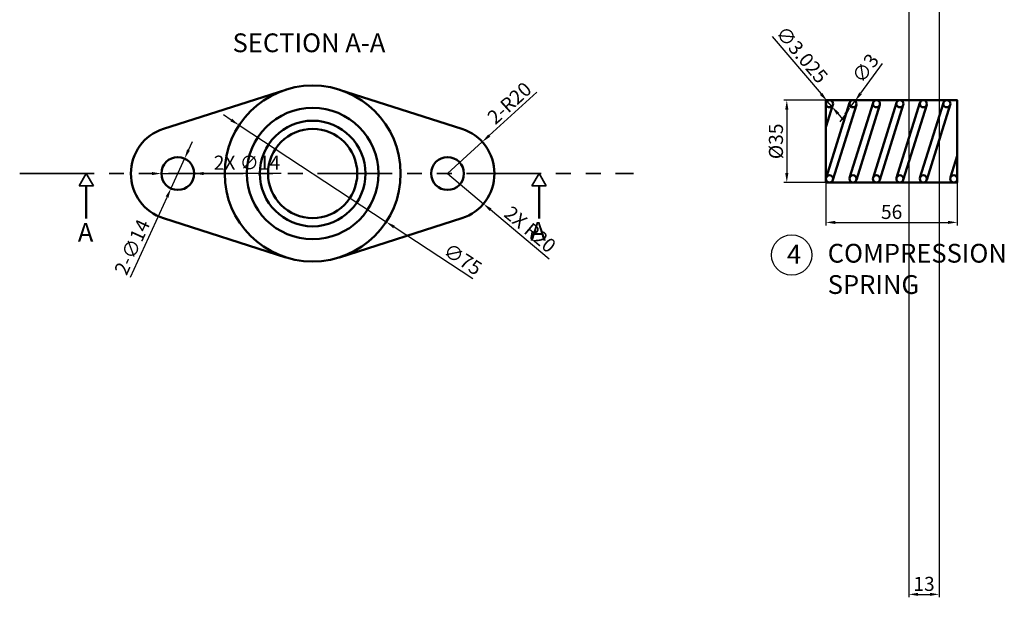
# Model space of a CAD drawing. Units: millimetres. Extents: x 4194 to 4882, y 3816 to 4286.
# Tile 1 of 3: x 4194 to 4614, y 3816 to 4062. Entities that reach past the tile are written whole.
import ezdxf

# ---------------------------------------------------------------- set-up
doc = ezdxf.new("R2010")
doc.units = ezdxf.units.MM
doc.linetypes.add('PHANTOM', pattern=[63.5, 31.75, -6.35, 6.35, -6.35, 6.35, -6.35])
for name, color, linetype, lineweight in [('M-DIMS', 2, 'Continuous', 25), ('M-OUTL', 7, 'Continuous', 50), ('M-SECT', 6, 'PHANTOM', 35), ('M-TEXT', 3, 'Continuous', 25)]:
    doc.layers.add(name, color=color, linetype=linetype, lineweight=lineweight)
doc.styles.get("Standard").update_dxf_attribs({"font": 'arial.ttf'})
doc.dimstyles.new('ISO-25', dxfattribs={"dimtxt": 6, "dimasz": 4, "dimexe": 1.25, "dimexo": 0.625, "dimtad": 1, "dimdec": 0, "dimtxsty": 'Standard', "dimcen": 2.5, "dimadec": 0, "dimazin": 0, "dimtfac": 1, "dimtdec": 0, "dimtmove": 0, "dimatfit": 3, "dimfxl": 1, "dimarcsym": 0})

# ---------------------------------------------------------------- blocks, each defined once
blk = doc.blocks.new('*D5')
at = {"layer": 'Defpoints', "color": 0, "transparency": 16777216}
for p in [(4264.77, 4003.28), (4258.94, 3990.55)]:
    blk.add_point(p, dxfattribs=at)
at = {"layer": 'M-DIMS', "color": 0, "lineweight": -2, "transparency": 16777216}
for p, q in [((4266.44, 4006.92), (4268.1, 4010.55)), ((4264.77, 4003.28), (4258.94, 3990.55)), ((4241.67, 3952.8), (4257.28, 3986.91))]:
    blk.add_line(p, q, dxfattribs=at)
at = {"layer": 'M-DIMS', "color": 0, "transparency": 16777216}
for points in [[(4265.83, 4007.19), (4267.04, 4006.64), (4264.77, 4003.28)], [(4256.67, 3987.19), (4257.89, 3986.63), (4258.94, 3990.55)]]:
    blk.add_solid(points, dxfattribs=at)
at = {"layer": 'M-DIMS', "color": 0, "transparency": 16777216, "insert": (4243.13, 3965.27), "char_height": 6, "attachment_point": 5, "rotation": 65.4036}
blk.add_mtext('2-∅14', dxfattribs=at)
blk = doc.blocks.new('*D6')
at = {"layer": 'Defpoints', "color": 0, "transparency": 16777216}
for p in [(4391.65, 4010.38), (4376.86, 3996.91)]:
    blk.add_point(p, dxfattribs=at)
at = {"layer": 'M-DIMS', "color": 0, "lineweight": -2, "transparency": 16777216}
for p, q in [((4414.9, 4031.53), (4394.61, 4013.07)), ((4376.86, 3996.91), (4391.65, 4010.38))]:
    blk.add_line(p, q, dxfattribs=at)
at = {"layer": 'M-DIMS', "color": 0, "transparency": 16777216}
blk.add_solid([(4394.16, 4013.56), (4395.06, 4012.57), (4391.65, 4010.38)], dxfattribs=at)
at = {"layer": 'M-DIMS', "color": 0, "transparency": 16777216, "insert": (4403.75, 4026.37), "char_height": 6, "attachment_point": 5, "rotation": 42.3036}
blk.add_mtext('2-R20', dxfattribs=at)
blk = doc.blocks.new('*D7')
at = {"layer": 'Defpoints', "color": 0, "transparency": 16777216}
for p in [(4288.01, 4017.5), (4350.7, 3976.33)]:
    blk.add_point(p, dxfattribs=at)
at = {"layer": 'M-DIMS', "color": 0, "lineweight": -2, "transparency": 16777216}
for p, q in [((4284.67, 4019.69), (4281.33, 4021.89)), ((4288.01, 4017.5), (4350.7, 3976.33)), ((4387.68, 3952.05), (4354.05, 3974.13))]:
    blk.add_line(p, q, dxfattribs=at)
at = {"layer": 'M-DIMS', "color": 0, "transparency": 16777216}
for points in [[(4285.04, 4020.25), (4284.3, 4019.14), (4288.01, 4017.5)], [(4354.41, 3974.69), (4353.68, 3973.58), (4350.7, 3976.33)]]:
    blk.add_solid(points, dxfattribs=at)
at = {"layer": 'M-DIMS', "color": 0, "transparency": 16777216, "insert": (4382.93, 3959.78), "char_height": 6, "attachment_point": 5, "rotation": 326.7072}
blk.add_mtext('∅75', dxfattribs=at)
blk = doc.blocks.new('*D30')
at = {"layer": 'Defpoints', "color": 0, "transparency": 16777216}
for p in [(4546.41, 4028.13), (4521.47, 3993.13), (4544.98, 3993.13)]:
    blk.add_point(p, dxfattribs=at)
at = {"layer": 'M-DIMS', "color": 0, "lineweight": -2, "transparency": 16777216}
for p, q in [((4545.79, 4028.13), (4520.22, 4028.13)), ((4521.47, 4024.13), (4521.47, 3997.13)), ((4544.35, 3993.13), (4520.22, 3993.13))]:
    blk.add_line(p, q, dxfattribs=at)
at = {"layer": 'M-DIMS', "color": 0, "transparency": 16777216}
for points in [[(4520.8, 4024.13), (4522.14, 4024.13), (4521.47, 4028.13)], [(4520.8, 3997.13), (4522.14, 3997.13), (4521.47, 3993.13)]]:
    blk.add_solid(points, dxfattribs=at)
at = {"layer": 'M-DIMS', "color": 0, "transparency": 16777216, "insert": (4517.62, 4010.63), "char_height": 6, "attachment_point": 5, "rotation": 90}
blk.add_mtext('%%C35', dxfattribs=at)
blk = doc.blocks.new('*D31')
at = {"layer": 'Defpoints', "color": 0, "transparency": 16777216}
for p in [(4594.15, 4010.63), (4538.15, 4007.59), (4594.15, 3976.09)]:
    blk.add_point(p, dxfattribs=at)
at = {"layer": 'M-DIMS', "color": 0, "lineweight": -2, "transparency": 16777216}
for p, q in [((4594.15, 4010.01), (4594.15, 3974.84)), ((4538.15, 4006.97), (4538.15, 3974.84)), ((4542.15, 3976.09), (4590.15, 3976.09))]:
    blk.add_line(p, q, dxfattribs=at)
at = {"layer": 'M-DIMS', "color": 0, "transparency": 16777216}
for points in [[(4542.15, 3976.76), (4542.15, 3975.42), (4538.15, 3976.09)], [(4590.15, 3976.76), (4590.15, 3975.42), (4594.15, 3976.09)]]:
    blk.add_solid(points, dxfattribs=at)
at = {"layer": 'M-DIMS', "color": 0, "transparency": 16777216, "insert": (4566.15, 3979.78), "char_height": 6, "attachment_point": 5}
blk.add_mtext('56', dxfattribs=at)
blk = doc.blocks.new('*D32')
at = {"layer": 'Defpoints', "color": 0, "transparency": 16777216}
for p in [(4548.78, 4025.41), (4550.56, 4027.85)]:
    blk.add_point(p, dxfattribs=at)
at = {"layer": 'M-DIMS', "color": 0, "lineweight": -2, "transparency": 16777216}
for p, q in [((4562.16, 4043.79), (4552.91, 4031.09)), ((4548.78, 4025.41), (4550.56, 4027.85)), ((4546.42, 4022.18), (4544.07, 4018.94))]:
    blk.add_line(p, q, dxfattribs=at)
at = {"layer": 'M-DIMS', "color": 0, "transparency": 16777216}
for points in [[(4552.37, 4031.48), (4553.45, 4030.69), (4550.56, 4027.85)], [(4545.88, 4022.57), (4546.96, 4021.78), (4548.78, 4025.41)]]:
    blk.add_solid(points, dxfattribs=at)
at = {"layer": 'M-DIMS', "color": 0, "transparency": 16777216, "insert": (4555.6, 4041.32), "char_height": 6, "attachment_point": 5, "rotation": 53.9324}
blk.add_mtext('∅3', dxfattribs=at)
blk = doc.blocks.new('SECTION-ARROW')
for p, q in [((3.04, 5.26), (0, 0)), ((3.04, 5.26), (6.07, 0)), ((6.07, 0), (0, 0))]:
    blk.add_line(p, q)
blk = doc.blocks.new('*D52')
at = {"layer": 'Defpoints', "color": 0, "transparency": 16777216}
for p in [(4586.46, 4107.44), (4573.46, 4094.44), (4586.46, 3817.63)]:
    blk.add_point(p, dxfattribs=at)
at = {"layer": 'M-DIMS', "color": 0, "lineweight": -2, "transparency": 16777216}
for p, q in [((4586.46, 4106.81), (4586.46, 3816.38)), ((4573.46, 4093.81), (4573.46, 3816.38)), ((4577.46, 3817.63), (4582.46, 3817.63))]:
    blk.add_line(p, q, dxfattribs=at)
at = {"layer": 'M-DIMS', "color": 0, "transparency": 16777216}
for points in [[(4577.46, 3818.3), (4577.46, 3816.97), (4573.46, 3817.63)], [(4582.46, 3818.3), (4582.46, 3816.97), (4586.46, 3817.63)]]:
    blk.add_solid(points, dxfattribs=at)
at = {"layer": 'M-DIMS', "color": 0, "transparency": 16777216, "insert": (4579.96, 3821.32), "char_height": 6, "attachment_point": 5}
blk.add_mtext('13', dxfattribs=at)
blk = doc.blocks.new('*D53')
at = {"layer": 'Defpoints', "color": 0, "transparency": 16777216}
for p in [(4376.86, 3996.91), (4392.16, 3984.03)]:
    blk.add_point(p, dxfattribs=at)
at = {"layer": 'M-DIMS', "color": 0, "lineweight": -2, "transparency": 16777216}
for p, q in [((4376.86, 3996.91), (4392.16, 3984.03)), ((4420.13, 3960.49), (4395.22, 3981.46))]:
    blk.add_line(p, q, dxfattribs=at)
at = {"layer": 'M-DIMS', "color": 0, "transparency": 16777216}
blk.add_solid([(4395.65, 3981.97), (4394.79, 3980.95), (4392.16, 3984.03)], dxfattribs=at)
at = {"layer": 'M-DIMS', "color": 0, "transparency": 16777216, "insert": (4411.58, 3972.51), "char_height": 6, "attachment_point": 5, "rotation": 319.9113}
blk.add_mtext('2X R20', dxfattribs=at)
blk = doc.blocks.new('*D54')
at = {"layer": 'Defpoints', "color": 0, "transparency": 16777216}
for p in [(4254.86, 3996.91), (4268.86, 3996.91)]:
    blk.add_point(p, dxfattribs=at)
at = {"layer": 'M-DIMS', "color": 0, "lineweight": -2, "transparency": 16777216}
for p, q in [((4250.86, 3996.91), (4246.86, 3996.91)), ((4254.86, 3996.91), (4268.86, 3996.91)), ((4305.88, 3996.91), (4272.86, 3996.91))]:
    blk.add_line(p, q, dxfattribs=at)
at = {"layer": 'M-DIMS', "color": 0, "transparency": 16777216}
for points in [[(4250.86, 3997.58), (4250.86, 3996.25), (4254.86, 3996.91)], [(4272.86, 3997.58), (4272.86, 3996.25), (4268.86, 3996.91)]]:
    blk.add_solid(points, dxfattribs=at)
at = {"layer": 'M-DIMS', "color": 0, "transparency": 16777216, "insert": (4291.37, 4000.77), "char_height": 6, "attachment_point": 5, "rotation": 359.9997}
blk.add_mtext('2X ∅14', dxfattribs=at)
blk = doc.blocks.new('*D57')
at = {"layer": 'Defpoints', "color": 0, "transparency": 16777216}
for p in [(4538.69, 4027.78), (4540.65, 4025.48)]:
    blk.add_point(p, dxfattribs=at)
at = {"layer": 'M-DIMS', "color": 0, "lineweight": -2, "transparency": 16777216}
for p, q in [((4515.29, 4055.23), (4536.09, 4030.83)), ((4540.65, 4025.48), (4538.69, 4027.78)), ((4543.24, 4022.44), (4545.84, 4019.39))]:
    blk.add_line(p, q, dxfattribs=at)
at = {"layer": 'M-DIMS', "color": 0, "transparency": 16777216}
for points in [[(4536.6, 4031.26), (4535.58, 4030.39), (4538.69, 4027.78)], [(4543.75, 4022.87), (4542.74, 4022), (4540.65, 4025.48)]]:
    blk.add_solid(points, dxfattribs=at)
at = {"layer": 'M-DIMS', "color": 0, "transparency": 16777216, "insert": (4527.33, 4047.05), "char_height": 6, "attachment_point": 5, "rotation": 310.4453}
blk.add_mtext('∅3.025', dxfattribs=at)

msp = doc.modelspace()

# ---------------------------------------------------------------- linework, layer by layer
at = {"layer": 'M-OUTL'}
for p, q in [((4307.9449, 4032.6351), (4255.771, 4015.9653)), ((4330.771, 4032.6351), (4382.9449, 4015.9653)), ((4538.2229, 4027.0821), (4538.1542, 4026.862)), ((4541.1104, 4026.1807), (4538.1542, 4016.711)), ((4548.2229, 4027.0821), (4538.2375, 3995.0945)), ((4551.1104, 4026.1807), (4541.1249, 3994.1931)), ((4558.2229, 4027.0821), (4548.2375, 3995.0945)), ((4561.1104, 4026.1807), (4551.1249, 3994.1931)), ((4568.2229, 4027.0821), (4558.2375, 3995.0945)), ((4571.1104, 4026.1807), (4561.1249, 3994.1931)), ((4578.2229, 4027.0821), (4568.2375, 3995.0945)), ((4581.1104, 4026.1807), (4571.1249, 3994.1931)), ((4588.2229, 4027.0821), (4578.2375, 3995.0945)), ((4591.1104, 4026.1807), (4581.1249, 3994.1931)), ((4591.287, 3995.3159), (4594.1542, 4004.501)), ((4222.8708, 3991.6564), (4222.8708, 3977.7143)), ((4415.8451, 3991.6564), (4415.8451, 3977.7143)), ((4307.9449, 3961.193), (4255.771, 3977.8628)), ((4330.771, 3961.193), (4382.9449, 3977.8628))]:
    msp.add_line(p, q, dxfattribs=at)
msp.add_lwpolyline([(4538.1542, 4028.1314), (4594.1542, 4028.1314), (4594.1542, 3993.1314), (4538.1542, 3993.1314)], close=True, dxfattribs=at)
for centre, radius in [((4319.358, 3996.914), 37.5), ((4539.6667, 4026.6314), 1.5124), ((4549.6667, 4026.6314), 1.5124), ((4559.6667, 4026.6314), 1.5124), ((4569.6667, 4026.6314), 1.5124), ((4579.6667, 4026.6314), 1.5124), ((4589.6667, 4026.6314), 1.5124), ((4319.358, 3996.914), 28), ((4319.358, 3996.914), 22.5), ((4319.358, 3996.914), 19), ((4261.858, 3996.914), 7), ((4376.858, 3996.914), 7), ((4539.6812, 3994.6438), 1.5124), ((4549.6812, 3994.6438), 1.5124), ((4559.6812, 3994.6438), 1.5124), ((4569.6812, 3994.6438), 1.5124), ((4579.6812, 3994.6438), 1.5124), ((4592.6418, 3994.6438), 1.5124)]:
    msp.add_circle(centre, radius, dxfattribs=at)
for centre, radius, start, end in [((4539.6667, 4026.6314), 1.5124, 342.663423, 180), ((4261.858, 3996.914), 20, 107.718932, 252.281068), ((4376.858, 3996.914), 20, 287.718932, 72.281068)]:
    msp.add_arc(centre, radius, start, end, dxfattribs=at)
at = {"layer": 'M-SECT'}
msp.add_line((4194.4762, 3996.914), (4456.1273, 3996.914), dxfattribs=at)
at = {"layer": 'M-TEXT'}
msp.add_circle((4523.548, 3962.2066), 8.6164, dxfattribs=at)

# ---------------------------------------------------------------- block references
at = {"layer": 'M-SECT', "rotation": 119.9999999999872}
msp.add_blockref('SECTION-ARROW', (4225.9065, 3991.657), dxfattribs=at)
at = {"layer": 'M-SECT'}
msp.add_blockref('SECTION-ARROW', (4412.81, 3991.656), dxfattribs=at)

# ---------------------------------------------------------------- texts
at = {"layer": 'M-TEXT', "char_height": 8, "attachment_point": 1}
for s, width, insert in [('SECTION A-A', 117.140838, (4285.2138, 4056.6039)), ('A', 8, (4219.2448, 3975.8547)), ('A', 8, (4412.1631, 3976.3338)), ('4', 8, (4521.5459, 3966.5448)), ('COMPRESSION \\PSPRING', 89.679929, (4538.8995, 3966.9548))]:
    msp.add_mtext_dynamic_manual_height_columns(s, width=width, gutter_width=12.5, heights=[0], dxfattribs=dict(at, insert=insert))

# ---------------------------------------------------------------- dimensions: what is measured, and where the dimension line sits
at = {"layer": 'M-DIMS'}
for base, p1, p2, override, picture, middle in [((4586.4627, 3817.6331), (4573.4627, 4094.4374), (4586.4627, 4107.4374), {"dimdec": 0, "dimlfac": 1, "dimrnd": 0, "dimzin": 0, "dimdsep": 46, "dimlunit": 2}, '*D52', (4579.9627, 3821.3236)), ((4594.1542, 3976.0886), (4538.1542, 4007.5949), (4594.1542, 4010.6314), {"dimclrd": 0, "dimclre": 0, "dimclrt": 0}, '*D31', (4566.1542, 3979.777))]:
    dim = msp.add_linear_dim(base=base, p1=p1, p2=p2, dimstyle='ISO-25', override=override, dxfattribs=at)
    dim.commit()
    dim.dimension.update_dxf_attribs({"geometry": picture, "text_midpoint": middle})
for p1, p2, override, picture, middle in [((4540.6478, 4025.4804), (4538.6855, 4027.7824), {"dimdec": 3, "dimlfac": 1, "dimrnd": 0, "dimzin": 0, "dimdsep": 46, "dimlunit": 2}, '*D57', (4524.391, 4044.5515)), ((4288.0126, 4017.4985), (4350.7033, 3976.3296), {"dimclrd": 0, "dimclre": 0, "dimclrt": 0}, '*D7', (4380.8178, 3956.5535))]:
    dim = msp.add_diameter_dim_2p(p1=p1, p2=p2, dimstyle='ISO-25', override=override, dxfattribs=at)
    dim.commit()
    dim.dimension.update_dxf_attribs({"geometry": picture, "text_midpoint": middle, "dimtype": 163})
dim = msp.add_diameter_dim_2p(p1=(4548.7762, 4025.4089), p2=(4550.5571, 4027.8539), dimstyle='ISO-25', override={"dimclrd": 0, "dimclre": 0, "dimclrt": 0}, dxfattribs=at)
dim.commit()
dim.dimension.update_dxf_attribs({"geometry": '*D32', "text_midpoint": (4555.5973, 4041.324)})
for mpoint, text, override, picture, middle in [((4391.6497, 4010.3752), '2-<>', {"dimclrd": 0, "dimclre": 0, "dimclrt": 0}, '*D6', (4403.7492, 4026.3734)), ((4392.1589, 3984.0346), '2X <>', {"dimdec": 0, "dimlfac": 1, "dimrnd": 0, "dimzin": 0, "dimdsep": 46, "dimlunit": 2}, '*D53', (4411.5799, 3972.5084))]:
    dim = msp.add_radius_dim(center=(4376.858, 3996.914), mpoint=mpoint, text=text, dimstyle='ISO-25', override=override, dxfattribs=at)
    dim.commit()
    dim.dimension.update_dxf_attribs({"geometry": picture, "text_midpoint": middle})
dim = msp.add_linear_dim(base=(4521.4713, 3993.1314), p1=(4546.4114, 4028.1314), p2=(4544.978, 3993.1314), angle=90, text='%%C<>', dimstyle='ISO-25', override={"dimclrd": 0, "dimclre": 0, "dimclrt": 0}, dxfattribs=at)
dim.commit()
dim.dimension.update_dxf_attribs({"geometry": '*D30', "text_midpoint": (4517.6151, 4010.6314)})
for p1, p2, text, override, picture, middle in [((4264.7715, 4003.2789), (4258.9444, 3990.5492), '2-<>', {"dimclrd": 0, "dimclre": 0, "dimclrt": 0}, '*D5', (4246.6383, 3963.6659)), ((4254.858, 3996.9141), (4268.858, 3996.914), '2X <>', {"dimdec": 0, "dimlfac": 1, "dimrnd": 0, "dimzin": 0, "dimdsep": 46, "dimlunit": 2}, '*D54', (4291.3697, 3996.9139))]:
    dim = msp.add_diameter_dim_2p(p1=p1, p2=p2, text=text, dimstyle='ISO-25', override=override, dxfattribs=at)
    dim.commit()
    dim.dimension.update_dxf_attribs({"geometry": picture, "text_midpoint": middle, "dimtype": 163})

doc.saveas('drawing.dxf')
